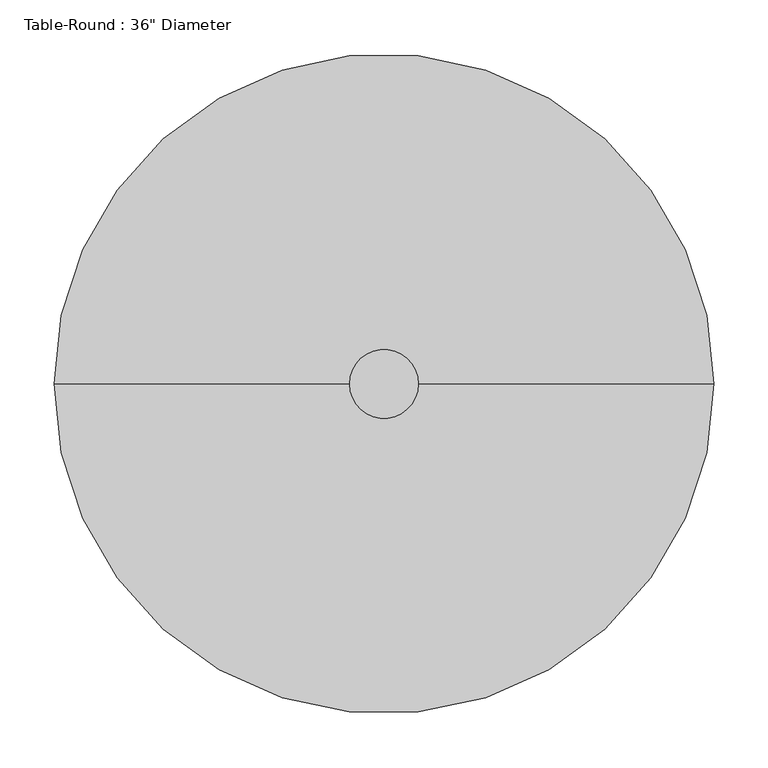
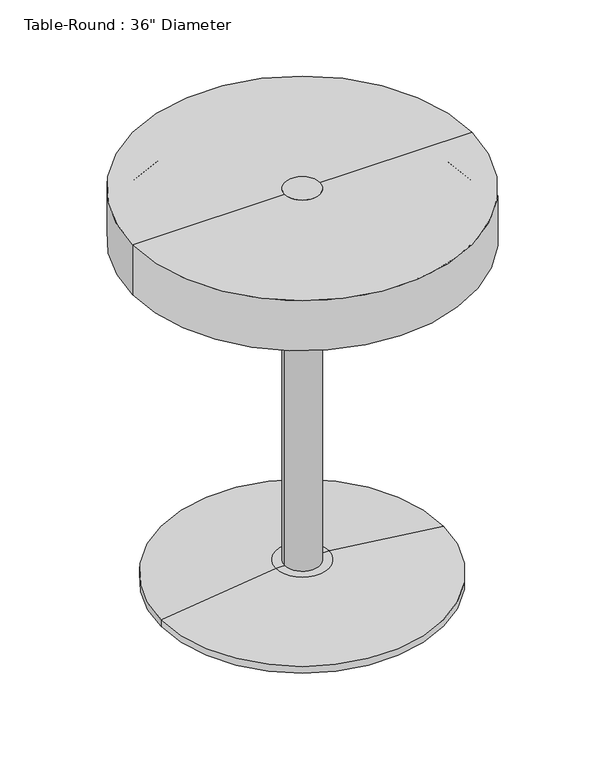
"""IFC4 building model written with IfcOpenShell, lengths in millimetres: furniture geometry."""

from ifc_helpers import new_model, si_unit, point, frame, origin, origin_2d, place, context, project, spatial, polyline, circle_curve, ellipse_curve, trimmed, segment, composite_curve, outline, extrude, source, transform, mapped, element, save
from ifc_brep_helpers import plane_surface, cylinder_surface, revolved_surface, advanced_brep


def furniture_1e21b0be(model_context):
    return source(origin(), model_context, "Body", "SolidModel", [
        extrude(outline(composite_curve([segment(trimmed(circle_curve(origin_2d(), 31.75), [point((-31.75, 0.0))], [point((31.75, 0.0))], False, "CARTESIAN"), True, "CONTINUOUS"), segment(trimmed(circle_curve(origin_2d(), 31.75), [point((31.75, 0.0))], [point((-31.75, 0.0))], False, "CARTESIAN"), True, "CONTINUOUS")], self_intersect=False)), frame((0.0, 0.0, 38.1), z_axis=(0.0, 0.0, 1.0), x_axis=(1.0, 0.0, 0.0)), (0.0, 0.0, 1.0), 704.85),
        advanced_brep(
        [(304.8, 0.0, 742.95), (-304.8, 0.0, 742.95), (0.0, 0.0, 742.95), (0.0, 0.0, 660.4), (-262.9011364, 0.0, 660.4), (262.9011364, 0.0, 660.4), (-299.5526659, 0.0, 653.9373465), (299.5526659, 0.0, 653.9373465), (-304.8, 0.0, 647.6838172), (304.8, 0.0, 647.6838172)],
        [
            (0, 1, circle_curve(frame((0.0, 0.0, 742.95), z_axis=(0.0, 0.0, 1.0), x_axis=(-1.0, 0.0, 0.0)), 304.8)),
            (1, 2),
            (2, 0),
            (1, 0, circle_curve(frame((0.0, 0.0, 742.95), z_axis=(0.0, 0.0, 1.0), x_axis=(-1.0, 0.0, 0.0)), 304.8)),
            (3, 4),
            (4, 5, circle_curve(frame((0.0, 0.0, 660.4), z_axis=(0.0, 0.0, -1.0), x_axis=(-1.0, 0.0, 0.0)), 262.9011364)),
            (5, 3),
            (5, 4, circle_curve(frame((0.0, 0.0, 660.4), z_axis=(0.0, 0.0, -1.0), x_axis=(-1.0, 0.0, 0.0)), 262.9011364)),
            (4, 6),
            (6, 7, circle_curve(frame((0.0, 0.0, 653.9373465), z_axis=(0.0, 0.0, -1.0), x_axis=(-1.0, 0.0, 0.0)), 299.5526659)),
            (7, 5),
            (7, 6, circle_curve(frame((0.0, 0.0, 653.9373465), z_axis=(0.0, 0.0, -1.0), x_axis=(-1.0, 0.0, 0.0)), 299.5526659)),
            (6, 8, circle_curve(frame((-298.45, 0.0, 647.6838172), z_axis=(0.0, -1.0, 0.0), x_axis=(1.0, 0.0, 0.0)), 6.35)),
            (8, 9, circle_curve(frame((0.0, 0.0, 647.6838172), z_axis=(0.0, 0.0, -1.0), x_axis=(-1.0, 0.0, 0.0)), 304.8)),
            (9, 7, circle_curve(frame((298.45, 0.0, 647.6838172), z_axis=(0.0, -1.0, 0.0), x_axis=(-1.0, 0.0, 0.0)), 6.35)),
            (9, 8, circle_curve(frame((0.0, 0.0, 647.6838172), z_axis=(0.0, 0.0, -1.0), x_axis=(-1.0, 0.0, 0.0)), 304.8)),
            (8, 1),
            (0, 9),
        ],
        [
            plane_surface(frame((0.0, 0.0, 742.95), z_axis=(0.0, 0.0, 1.0), x_axis=(-1.0, 0.0, 0.0))),
            plane_surface(frame((0.0, 0.0, 660.4), z_axis=(0.0, 0.0, -1.0), x_axis=(-1.0, 0.0, 0.0))),
            revolved_surface(polyline([(-299.5526659, 0.0, 653.9373465), (-262.9011364, 0.0, 660.4)]), (0.0, 0.0, 736.6), (0.0, 0.0, -1.0)),
            revolved_surface(trimmed(ellipse_curve(frame((-298.45, 0.0, 647.6838172), z_axis=(0.0, 1.0, 0.0), x_axis=(1.0, 0.0, 0.0)), 6.35, 6.35), [point((-304.8, 0.0, 647.6838172))], [point((-299.5526659, 0.0, 653.9373465))], True, "CARTESIAN"), (0.0, 0.0, 736.6), (0.0, 0.0, -1.0)),
            cylinder_surface(frame((0.0, 0.0, 736.6), z_axis=(0.0, 0.0, -1.0), x_axis=(-1.0, 0.0, 0.0)), 304.8),
        ],
        [
            (0, [[1, 2, 3]]),
            (0, [[4, -3, -2]]),
            (1, [[5, 6, 7]]),
            (1, [[-7, 8, -5]]),
            (2, [[-6, 9, 10, 11]]),
            (2, [[-8, -11, 12, -9]]),
            (3, [[-10, 13, 14, 15]]),
            (3, [[-12, -15, 16, -13]]),
            (4, [[-14, 17, -1, 18]]),
            (4, [[-16, -18, -4, -17]]),
        ],
    ),
        advanced_brep(
        [(0.0, 0.0, 0.0), (-254.0, 0.0, 0.0), (254.0, 0.0, 0.0), (47.625, 0.0, 38.1), (-47.625, 0.0, 38.1), (0.0, 0.0, 38.1), (254.0, 0.0, 12.7), (-254.0, 0.0, 12.7)],
        [
            (0, 1),
            (1, 2, circle_curve(frame((0.0, 0.0, 0.0), z_axis=(0.0, 0.0, -1.0), x_axis=(-1.0, 0.0, 0.0)), 254.0)),
            (2, 0),
            (2, 1, circle_curve(frame((0.0, 0.0, 0.0), z_axis=(0.0, 0.0, -1.0), x_axis=(-1.0, 0.0, 0.0)), 254.0)),
            (3, 4, circle_curve(frame((0.0, 0.0, 38.1), z_axis=(0.0, 0.0, 1.0), x_axis=(-1.0, 0.0, 0.0)), 47.625)),
            (4, 5),
            (5, 3),
            (4, 3, circle_curve(frame((0.0, 0.0, 38.1), z_axis=(0.0, 0.0, 1.0), x_axis=(-1.0, 0.0, 0.0)), 47.625)),
            (6, 7, circle_curve(frame((0.0, 0.0, 12.7), z_axis=(0.0, 0.0, 1.0), x_axis=(-1.0, 0.0, 0.0)), 254.0)),
            (7, 4),
            (3, 6),
            (7, 6, circle_curve(frame((0.0, 0.0, 12.7), z_axis=(0.0, 0.0, 1.0), x_axis=(-1.0, 0.0, 0.0)), 254.0)),
            (1, 7),
            (6, 2),
        ],
        [
            plane_surface(frame((0.0, 0.0, 0.0), z_axis=(0.0, 0.0, -1.0), x_axis=(-1.0, 0.0, 0.0))),
            plane_surface(frame((0.0, 0.0, 38.1), z_axis=(0.0, 0.0, 1.0), x_axis=(-1.0, 0.0, 0.0))),
            revolved_surface(polyline([(-47.625, 0.0, 38.1), (-254.0, 0.0, 12.7)]), (0.0, 0.0, 215.9), (0.0, 0.0, -1.0)),
            cylinder_surface(frame((0.0, 0.0, 215.9), z_axis=(0.0, 0.0, -1.0), x_axis=(-1.0, 0.0, 0.0)), 254.0),
        ],
        [
            (0, [[1, 2, 3]]),
            (0, [[-3, 4, -1]]),
            (1, [[5, 6, 7]]),
            (1, [[8, -7, -6]]),
            (2, [[9, 10, -5, 11]]),
            (2, [[12, -11, -8, -10]]),
            (3, [[-2, 13, -9, 14]]),
            (3, [[-4, -14, -12, -13]]),
        ],
    ),
    ])


if __name__ == "__main__":
    model = new_model("IFC4")
    model_context = context("Model", 3, world=origin())
    ifc_project = project(units=[si_unit("LENGTHUNIT", "METRE", prefix="MILLI")], contexts=[model_context])
    site = spatial("IfcSite", under=ifc_project)
    building = spatial("IfcBuilding", under=site)
    placement = place(None, origin())
    furniture_shape = furniture_1e21b0be(model_context)
    element("IfcFurniture", 1, ObjectType="Table-Round : 36\" Diameter", at=placement, inside=building, context=model_context, shape_type="MappedRepresentation", body=[
        mapped(furniture_shape, transform((0.0, 0.0, 0.0), x_axis=(1.0, 0.0, 0.0), y_axis=(0.0, 1.0, 0.0), z_axis=(0.0, 0.0, 1.0))),
    ])
    save(model, "model.ifc")

# Revit data of these elements
# Type "Table-Round : 36\" Diameter"
#   Assembly Code = "E2020200"
#   Base Radius = 0' - 10"
#   Height = 2' - 2"
#   Radius = 1' - 0"
#   Base Material = Steel, Chrome Plated
#   Top Material = Birch
#   Default Elevation = 0
# Element 1 (IfcFurniture, "Table-Round : 36\" Diameter")
#   Materials on its faces: "Steel, Chrome Plated", "Birch"
# Materials
#   "Steel, Chrome Plated": class "Metal", colour RGB 17 17 17, transparency 0, Description = "Chromiuim plated steel", Cost = 0
#   "Birch": class "Wood", colour RGB 210 159 95, transparency 0, Description = "Betula Alleghaniensis", Cost = 0
